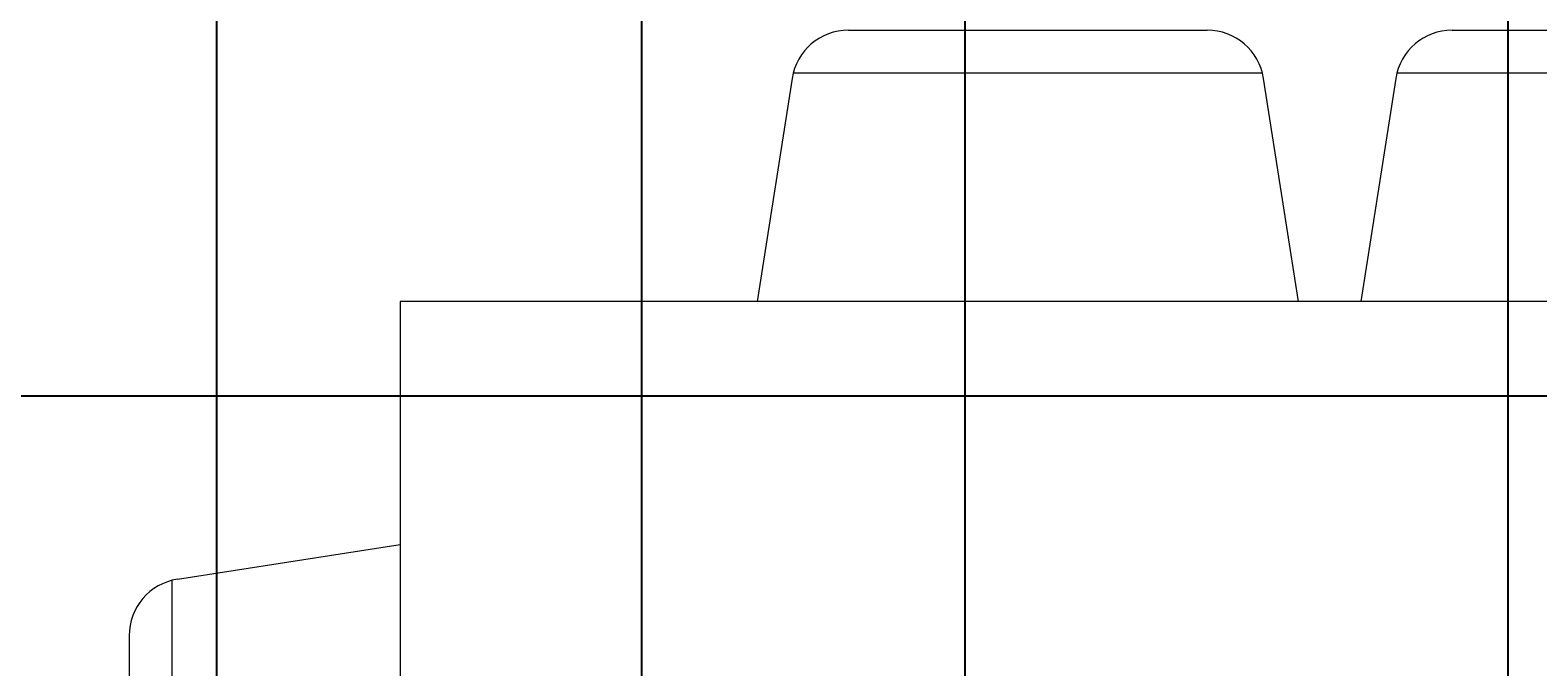
# Model space of a CAD drawing. Units: inches. Extents: x 2231 to 2461, y 2045 to 2455.
# Tile 26 of 95: x 2326 to 2361, y 2144 to 2159. Entities that reach past the tile are written whole.
import ezdxf

# ---------------------------------------------------------------- set-up
doc = ezdxf.new("R2010")
doc.units = ezdxf.units.IN
doc.layers.add('A-ANNO-DIMS', color=2, linetype='Continuous', lineweight=18)
doc.layers.add('A-FURN', color=9, linetype='Continuous', lineweight=18)
doc.styles.get("Standard").update_dxf_attribs({"font": 'arial.ttf'})
doc.dimstyles.get("Standard").update_dxf_attribs({"dimtxt": 0.18, "dimasz": 0.18, "dimexe": 0.18, "dimexo": 0.0625, "dimgap": 0.09, "dimtad": 0, "dimtih": 1, "dimtoh": 1, "dimdec": 4, "dimzin": 0, "dimdsep": 46, "dimtxsty": 'Standard', "dimcen": 0.09, "dimadec": 0, "dimazin": 0, "dimtfac": 1, "dimtdec": 4, "dimtofl": 0, "dimtmove": 0, "dimatfit": 3, "dimfxl": 1, "dimtolj": 1, "dimtzin": 0, "dimarcsym": 0})

# ---------------------------------------------------------------- blocks, each defined once
blk = doc.blocks.new('Dining Set - 36 x 72 in.')
for p, q in [((-20.288, 27.5), (-7.712, 27.5)), ((0.874, 27.5), (13.451, 27.5)), ((-22.23, 26), (-5.761, 26)), ((-1.068, 26), (15.402, 26)), ((-22.264, 25.809), (-23.485, 17.998)), ((-4.515, 17.998), (-5.736, 25.809)), ((-1.102, 25.809), (-2.322, 17.998)), ((-36, 18), (-36, -18)), ((-4.062, 18), (-36, 18)), ((29.162, 18), (-4.062, 18)), ((-43.809, 8.264), (-35.998, 9.485)), ((-44, 8.23), (-44, -8.239)), ((-45.5, 6.288), (-45.5, -6.288))]:
    blk.add_line(p, q)
for centre, start, end in [((-20.288, 25.5), 90, 171.1198), ((-7.712, 25.5), 8.881, 90), ((0.874, 25.5), 90, 171.1198), ((-43.5, 6.288), 98.8806, 180)]:
    blk.add_arc(centre, 2, start, end)
blk = doc.blocks.new('*D51')
at = {"layer": 'A-ANNO-DIMS', "color": 0, "lineweight": -2, "transparency": 16777216}
for p, q in [((2258.794, 2306.77), (2258.794, 2044.803)), ((2330.794, 2306.77), (2330.794, 2044.803)), ((2258.974, 2044.983), (2294.576, 2044.983)), ((2330.614, 2044.983), (2295.011, 2044.983))]:
    blk.add_line(p, q, dxfattribs=at)
at = {"layer": 'A-ANNO-DIMS', "color": 0, "transparency": 16777216}
for points in [[(2258.974, 2045.013), (2258.974, 2044.953), (2258.794, 2044.983)], [(2330.614, 2045.013), (2330.614, 2044.953), (2330.794, 2044.983)]]:
    blk.add_solid(points, dxfattribs=at)
at = {"layer": 'Defpoints', "color": 0, "transparency": 16777216}
for p in [(2258.794, 2306.833), (2330.794, 2306.833), (2330.794, 2044.983)]:
    blk.add_point(p, dxfattribs=at)
at = {"layer": 'A-ANNO-DIMS', "color": 0, "transparency": 16777216, "insert": (2294.794, 2044.983), "char_height": 0.18, "attachment_point": 5}
blk.add_mtext('\\A1;72', dxfattribs=at)
blk = doc.blocks.new('*D52')
at = {"layer": 'A-ANNO-DIMS', "color": 0, "lineweight": -2, "transparency": 16777216}
for p, q in [((2330.794, 2306.77), (2330.794, 2044.803)), ((2360.794, 2306.77), (2360.794, 2044.803)), ((2330.974, 2044.983), (2345.575, 2044.983)), ((2360.614, 2044.983), (2346.012, 2044.983))]:
    blk.add_line(p, q, dxfattribs=at)
at = {"layer": 'A-ANNO-DIMS', "color": 0, "transparency": 16777216}
for points in [[(2330.974, 2045.013), (2330.974, 2044.953), (2330.794, 2044.983)], [(2360.614, 2045.013), (2360.614, 2044.953), (2360.794, 2044.983)]]:
    blk.add_solid(points, dxfattribs=at)
at = {"layer": 'Defpoints', "color": 0, "transparency": 16777216}
for p in [(2330.794, 2306.833), (2360.794, 2306.833), (2360.794, 2044.983)]:
    blk.add_point(p, dxfattribs=at)
at = {"layer": 'A-ANNO-DIMS', "color": 0, "transparency": 16777216, "insert": (2345.794, 2044.983), "char_height": 0.18, "attachment_point": 5}
blk.add_mtext('\\A1;30', dxfattribs=at)
blk = doc.blocks.new('*D60')
at = {"layer": 'A-ANNO-DIMS', "color": 0, "lineweight": -2, "transparency": 16777216}
for p, q in [((2432.731, 2182.833), (2230.981, 2182.833)), ((2231.161, 2182.653), (2231.161, 2166.906)), ((2231.161, 2150.795), (2231.161, 2166.542)), ((2432.731, 2150.615), (2230.981, 2150.615))]:
    blk.add_line(p, q, dxfattribs=at)
at = {"layer": 'A-ANNO-DIMS', "color": 0, "transparency": 16777216}
for points in [[(2231.131, 2182.653), (2231.191, 2182.653), (2231.161, 2182.833)], [(2231.131, 2150.795), (2231.191, 2150.795), (2231.161, 2150.615)]]:
    blk.add_solid(points, dxfattribs=at)
at = {"layer": 'Defpoints', "color": 0, "transparency": 16777216}
for p in [(2231.161, 2182.833), (2432.794, 2182.833), (2432.794, 2150.615)]:
    blk.add_point(p, dxfattribs=at)
at = {"layer": 'A-ANNO-DIMS', "color": 0, "transparency": 16777216, "insert": (2231.161, 2166.724), "char_height": 0.18, "attachment_point": 5}
blk.add_mtext('\\A1;32.22', dxfattribs=at)
blk = doc.blocks.new('*D65')
at = {"layer": 'A-ANNO-DIMS', "color": 0, "lineweight": -2, "transparency": 16777216}
for p, q in [((2285.635, 2189.285), (2285.635, 2044.803)), ((2340.667, 2189.285), (2340.667, 2044.803)), ((2285.815, 2044.983), (2312.758, 2044.983)), ((2340.487, 2044.983), (2313.545, 2044.983))]:
    blk.add_line(p, q, dxfattribs=at)
at = {"layer": 'A-ANNO-DIMS', "color": 0, "transparency": 16777216}
for points in [[(2285.815, 2045.013), (2285.815, 2044.953), (2285.635, 2044.983)], [(2340.487, 2045.013), (2340.487, 2044.953), (2340.667, 2044.983)]]:
    blk.add_solid(points, dxfattribs=at)
at = {"layer": 'Defpoints', "color": 0, "transparency": 16777216}
for p in [(2285.635, 2189.348), (2340.667, 2189.348), (2340.667, 2044.983)]:
    blk.add_point(p, dxfattribs=at)
at = {"layer": 'A-ANNO-DIMS', "color": 0, "transparency": 16777216, "insert": (2313.151, 2044.983), "char_height": 0.18, "attachment_point": 5}
blk.add_mtext('\\A1;55.03', dxfattribs=at)
blk = doc.blocks.new('*D66')
at = {"layer": 'A-ANNO-DIMS', "color": 0, "lineweight": -2, "transparency": 16777216}
for p, q in [((2348.189, 2096.895), (2348.189, 2454.645)), ((2408.794, 2096.895), (2408.794, 2454.645)), ((2348.369, 2454.465), (2378.167, 2454.465)), ((2408.614, 2454.465), (2378.815, 2454.465))]:
    blk.add_line(p, q, dxfattribs=at)
at = {"layer": 'A-ANNO-DIMS', "color": 0, "transparency": 16777216}
for points in [[(2348.369, 2454.495), (2348.369, 2454.435), (2348.189, 2454.465)], [(2408.614, 2454.495), (2408.614, 2454.435), (2408.794, 2454.465)]]:
    blk.add_solid(points, dxfattribs=at)
at = {"layer": 'Defpoints', "color": 0, "transparency": 16777216}
for p in [(2408.794, 2454.465), (2348.189, 2096.833), (2408.794, 2096.833)]:
    blk.add_point(p, dxfattribs=at)
at = {"layer": 'A-ANNO-DIMS', "color": 0, "transparency": 16777216, "insert": (2378.491, 2454.465), "char_height": 0.18, "attachment_point": 5}
blk.add_mtext('\\A1;60.6', dxfattribs=at)
blk = doc.blocks.new('*D69')
at = {"layer": 'A-ANNO-DIMS', "color": 0, "lineweight": -2, "transparency": 16777216}
for p, q in [((2340.667, 2189.285), (2340.667, 2044.803)), ((2394.794, 2186.77), (2394.794, 2044.803)), ((2340.847, 2044.983), (2367.337, 2044.983)), ((2394.614, 2044.983), (2368.124, 2044.983))]:
    blk.add_line(p, q, dxfattribs=at)
at = {"layer": 'A-ANNO-DIMS', "color": 0, "transparency": 16777216}
for points in [[(2340.847, 2045.013), (2340.847, 2044.953), (2340.667, 2044.983)], [(2394.614, 2045.013), (2394.614, 2044.953), (2394.794, 2044.983)]]:
    blk.add_solid(points, dxfattribs=at)
at = {"layer": 'Defpoints', "color": 0, "transparency": 16777216}
for p in [(2340.667, 2189.348), (2394.794, 2186.833), (2394.794, 2044.983)]:
    blk.add_point(p, dxfattribs=at)
at = {"layer": 'A-ANNO-DIMS', "color": 0, "transparency": 16777216, "insert": (2367.73, 2044.983), "char_height": 0.18, "attachment_point": 5}
blk.add_mtext('\\A1;54.13', dxfattribs=at)

msp = doc.modelspace()

# ---------------------------------------------------------------- block references
at = {"layer": 'A-FURN', "xscale": 0.6627357546055535, "yscale": 0.6627357546055535, "zscale": 0.6627357546055535}
msp.add_blockref('Dining Set - 36 x 72 in.', (2358.9199, 2140.8902), dxfattribs=at)

# ---------------------------------------------------------------- dimensions: what is measured, and where the dimension line sits
at = {"layer": 'A-ANNO-DIMS'}
for base, p1, p2, override, picture, middle in [((2408.7935, 2454.4653), (2348.1888, 2096.8328), (2408.7935, 2096.8328), {"dimdec": 1, "dimlfac": 1, "dimrnd": 0, "dimzin": 0, "dimdsep": 46, "dimlunit": 2}, '*D66', (2378.4912, 2454.4653)), ((2330.7935, 2044.9825), (2258.7935, 2306.8328), (2330.7935, 2306.8328), {"dimdec": 0, "dimlfac": 1, "dimrnd": 0, "dimzin": 0, "dimdsep": 46, "dimlunit": 2}, '*D51', (2294.7935, 2044.9825)), ((2360.7935, 2044.9825), (2330.7935, 2306.8328), (2360.7935, 2306.8328), {"dimdec": 0, "dimlfac": 1, "dimrnd": 0, "dimzin": 0, "dimdsep": 46, "dimlunit": 2}, '*D52', (2345.7935, 2044.9825)), ((2340.6673, 2044.9825), (2285.6353, 2189.3477), (2340.6673, 2189.3477), {"dimdec": 2, "dimlfac": 1, "dimrnd": 0, "dimzin": 0, "dimdsep": 46, "dimlunit": 2}, '*D65', (2313.1513, 2044.9825)), ((2394.7935, 2044.9825), (2340.6673, 2189.3477), (2394.7935, 2186.8328), {"dimdec": 2, "dimlfac": 1, "dimrnd": 0, "dimzin": 0, "dimdsep": 46, "dimlunit": 2}, '*D69', (2367.7304, 2044.9825))]:
    dim = msp.add_linear_dim(base=base, p1=p1, p2=p2, dimstyle='Standard', override=override, dxfattribs=at)
    dim.commit()
    dim.dimension.update_dxf_attribs({"geometry": picture, "text_midpoint": middle})
dim = msp.add_linear_dim(base=(2231.161, 2182.8328), p1=(2432.7935, 2150.6145), p2=(2432.7935, 2182.8328), angle=90, dimstyle='Standard', override={"dimdec": 2, "dimlfac": 1, "dimrnd": 0, "dimzin": 0, "dimdsep": 46, "dimlunit": 2}, dxfattribs=at)
dim.commit()
dim.dimension.update_dxf_attribs({"geometry": '*D60', "text_midpoint": (2231.161, 2166.7237)})

doc.saveas('drawing.dxf')
